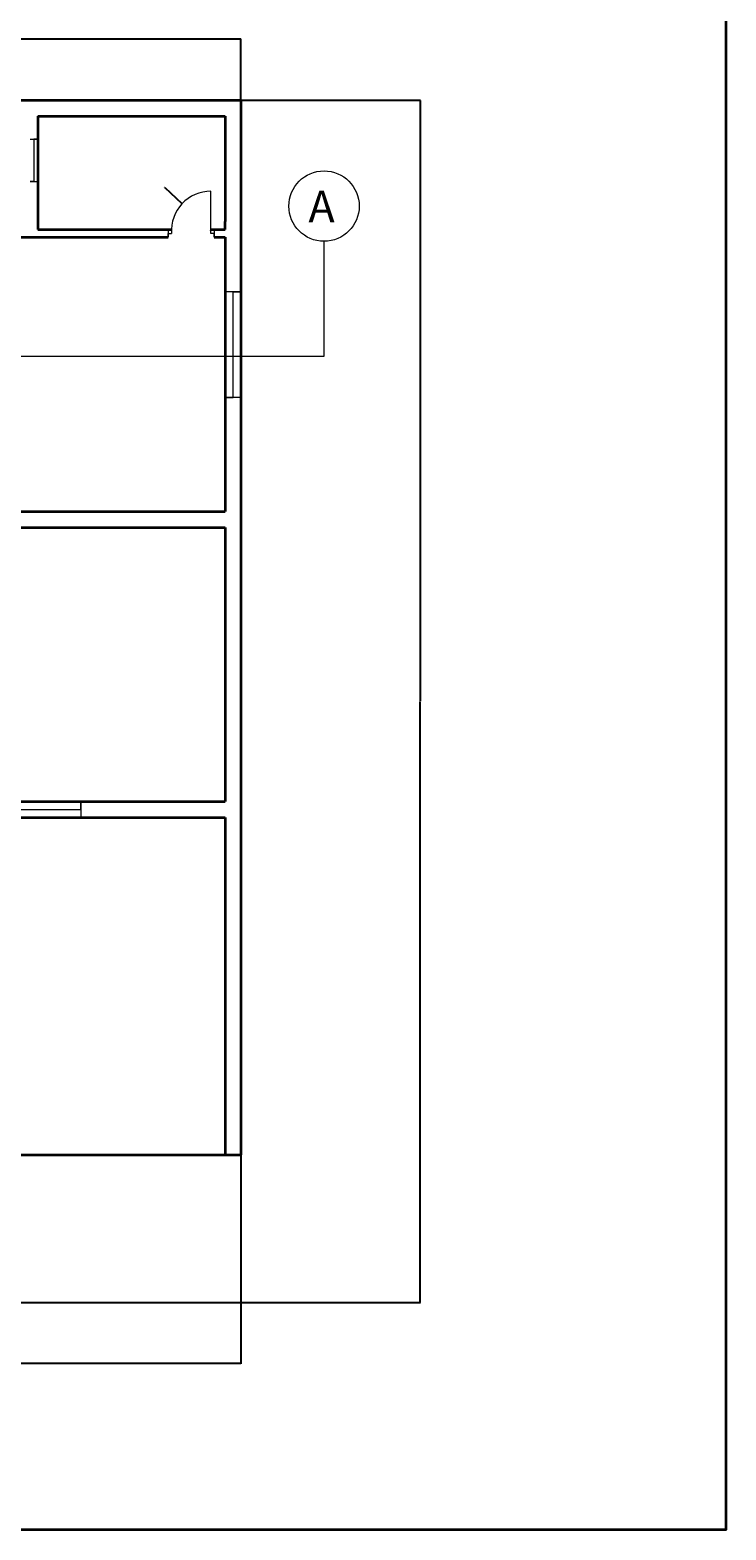
# Model space of a CAD drawing. Units: inches. Extents: x 2014 to 3678, y 870 to 2323.
# Tile 6 of 7: x 3282 to 3678, y 870 to 1723. Entities that reach past the tile are written whole.
import ezdxf

# ---------------------------------------------------------------- set-up
doc = ezdxf.new("R2010")
doc.units = ezdxf.units.IN
for name, color, linetype, lineweight in [('A-ANNO-DIMS', 2, 'Continuous', 18), ('A-ANNO-SYMB', 2, 'Continuous', 18), ('A-ANNO-TTLB', 7, 'Continuous', 35), ('A-DOOR', 3, 'Continuous', 18), ('A-GLAZ', 4, 'Continuous', 18), ('A-SITE', 8, 'Continuous', 25), ('A-WALL', 7, 'Continuous', 35)]:
    doc.layers.add(name, color=color, linetype=linetype, lineweight=lineweight)
doc.styles.get("Standard").update_dxf_attribs({"font": 'arial.ttf'})
doc.dimstyles.get("Standard").update_dxf_attribs({"dimtxt": 0.18, "dimasz": 0.18, "dimexe": 0.18, "dimexo": 0.0625, "dimgap": 0.09, "dimtad": 0, "dimtih": 1, "dimtoh": 1, "dimdec": 4, "dimzin": 0, "dimdsep": 46, "dimtxsty": 'Standard', "dimcen": 0.09, "dimadec": 0, "dimazin": 0, "dimtfac": 1, "dimtdec": 4, "dimtofl": 0, "dimtmove": 0, "dimatfit": 3, "dimfxl": 1, "dimtolj": 1, "dimtzin": 0, "dimarcsym": 0})

# ---------------------------------------------------------------- blocks, each defined once
blk = doc.blocks.new('DOOR-BATH-EAST-24')
for p, q in [((24.34, 2.25), (24.34, 26.25)), ((0, 4.5), (0, 0)), ((0, 0), (0, 2.25)), ((0, 2.25), (2, 2.25)), ((26.34, 2.25), (24.34, 2.25)), ((26.34, 4.5), (26.34, 0)), ((26.34, 0), (26.34, 2.25))]:
    blk.add_line(p, q)
blk.add_arc((24.34, 3.85), 22.4, 90, 184.10271)
blk = doc.blocks.new('WIN-60')
for p, q in [((0, 9), (0, 0)), ((60, 4.5), (60, 9)), ((60, 9), (60, 0)), ((0, 0), (0, 4.5)), ((0, 4.5), (60, 4.5))]:
    blk.add_line(p, q)
blk = doc.blocks.new('VENT-24')
for p, q in [((0, 24), (4.5, 24)), ((4.5, 24), (2.25, 24)), ((2.25, 24), (2.25, 0)), ((2.25, 0), (0, 0)), ((0, 0), (4.5, 0))]:
    blk.add_line(p, q)
blk = doc.blocks.new('*D91')
at = {"layer": 'A-ANNO-DIMS', "color": 0, "lineweight": -2, "transparency": 16777216}
for p, q in [((2848.67, 1683.23), (2848.67, 1718)), ((2848.85, 1717.82), (3125.03, 1717.82)), ((3401.99, 1717.82), (3125.82, 1717.82)), ((3402.17, 1683.23), (3402.17, 1718))]:
    blk.add_line(p, q, dxfattribs=at)
at = {"layer": 'A-ANNO-DIMS', "color": 0, "transparency": 16777216}
for points in [[(2848.85, 1717.85), (2848.85, 1717.79), (2848.67, 1717.82)], [(3401.99, 1717.85), (3401.99, 1717.79), (3402.17, 1717.82)]]:
    blk.add_solid(points, dxfattribs=at)
at = {"layer": 'Defpoints', "color": 0, "transparency": 16777216}
for p in [(3402.17, 1717.82), (2848.67, 1683.17), (3402.17, 1683.17)]:
    blk.add_point(p, dxfattribs=at)
at = {"layer": 'A-ANNO-DIMS', "color": 0, "transparency": 16777216, "insert": (3125.42, 1717.82), "char_height": 0.18, "attachment_point": 5}
blk.add_mtext('\\A1;553.5', dxfattribs=at)
blk = doc.blocks.new('*D92')
at = {"layer": 'A-ANNO-DIMS', "color": 0, "lineweight": -2, "transparency": 16777216}
for p, q in [((3402.23, 1683.17), (3504.23, 1683.17)), ((3504.05, 1682.99), (3504.05, 1341.35)), ((3504.05, 999.35), (3504.05, 1340.98)), ((3402.23, 999.17), (3504.23, 999.17))]:
    blk.add_line(p, q, dxfattribs=at)
at = {"layer": 'A-ANNO-DIMS', "color": 0, "transparency": 16777216}
for points in [[(3504.02, 1682.99), (3504.08, 1682.99), (3504.05, 1683.17)], [(3504.02, 999.35), (3504.08, 999.35), (3504.05, 999.17)]]:
    blk.add_solid(points, dxfattribs=at)
at = {"layer": 'Defpoints', "color": 0, "transparency": 16777216}
for p in [(3402.17, 1683.17), (3504.05, 1683.17), (3402.17, 999.17)]:
    blk.add_point(p, dxfattribs=at)
at = {"layer": 'A-ANNO-DIMS', "color": 0, "transparency": 16777216, "insert": (3504.05, 1341.17), "char_height": 0.18, "attachment_point": 5}
blk.add_mtext('\\A1;684', dxfattribs=at)
blk = doc.blocks.new('*D99')
at = {"layer": 'A-ANNO-DIMS', "color": 0, "lineweight": -2, "transparency": 16777216}
for p, q in [((3145.67, 999.1), (3145.67, 964.34)), ((3402.17, 999.1), (3402.17, 964.34)), ((3145.85, 964.52), (3273.53, 964.52)), ((3401.99, 964.52), (3274.32, 964.52))]:
    blk.add_line(p, q, dxfattribs=at)
at = {"layer": 'A-ANNO-DIMS', "color": 0, "transparency": 16777216}
for points in [[(3145.85, 964.55), (3145.85, 964.49), (3145.67, 964.52)], [(3401.99, 964.55), (3401.99, 964.49), (3402.17, 964.52)]]:
    blk.add_solid(points, dxfattribs=at)
at = {"layer": 'Defpoints', "color": 0, "transparency": 16777216}
for p in [(3145.67, 999.17), (3402.17, 999.17), (3402.17, 964.52)]:
    blk.add_point(p, dxfattribs=at)
at = {"layer": 'A-ANNO-DIMS', "color": 0, "transparency": 16777216, "insert": (3273.92, 964.52), "char_height": 0.18, "attachment_point": 5}
blk.add_mtext('\\A1;256.5', dxfattribs=at)
blk = doc.blocks.new('*D131')
at = {"layer": 'A-ANNO-DIMS', "color": 0, "lineweight": -2, "transparency": 16777216}
for p, q in [((3358.59, 1633.43), (3358.77, 1633.43)), ((3358.77, 1633.43), (3368.48, 1624.4)), ((3384.91, 1609.02), (3385.09, 1609.02)), ((3385, 1608.93), (3385, 1609.11))]:
    blk.add_line(p, q, dxfattribs=at)
at = {"layer": 'A-ANNO-DIMS', "color": 0, "transparency": 16777216}
blk.add_solid([(3368.5, 1624.42), (3368.46, 1624.38), (3368.61, 1624.28)], dxfattribs=at)
at = {"layer": 'Defpoints', "color": 0, "transparency": 16777216}
for p in [(3368.61, 1624.28), (3385, 1609.02)]:
    blk.add_point(p, dxfattribs=at)
at = {"layer": 'A-ANNO-DIMS', "color": 0, "transparency": 16777216, "insert": (3358.04, 1633.43), "char_height": 0.18, "attachment_point": 5}
blk.add_mtext('\\A1;R22.398', dxfattribs=at)

msp = doc.modelspace()

# ---------------------------------------------------------------- linework, layer by layer
at = {"layer": 'A-ANNO-SYMB'}
for p, q in [((3449.5026, 1537.5002), (3449.5026, 1602.9033)), ((2813.1731, 1537.5002), (3449.5026, 1537.5002))]:
    msp.add_line(p, q, dxfattribs=at)
msp.add_circle((3449.391, 1622.9101), 20.0072, dxfattribs=at)
at = {"layer": 'A-ANNO-TTLB'}
msp.add_lwpolyline([(2014.0556, 2323.3638), (3678.0069, 2323.3638), (3678.0069, 869.855), (2014.0556, 869.855)], close=True, dxfattribs=at)
at = {"layer": 'A-SITE'}
for p, q in [((3402.1718, 1083.1655), (3402.1718, 999.1655)), ((3402.1718, 999.1655), (2848.6718, 999.1655))]:
    msp.add_line(p, q, dxfattribs=at)
at = {"layer": 'A-WALL'}
for p, q in [((2848.6718, 1683.1655), (3402.1718, 1683.1655)), ((2848.6718, 1683.1655), (3402.1718, 1683.1655)), ((3402.1718, 1683.1655), (3402.1718, 1083.1655)), ((3286.6718, 1674.1655), (3393.1718, 1674.1655)), ((3286.6718, 1674.1655), (3286.6718, 1614.1655)), ((3393.1718, 1674.1655), (3393.1718, 1614.1655)), ((3286.6718, 1614.1655), (3286.6718, 1609.6655)), ((3393.1718, 1609.6655), (3393.1718, 1614.1655)), ((3216.1718, 1605.1655), (3360.6647, 1605.1655)), ((3286.6718, 1609.6655), (3362.6166, 1609.6655)), ((3385.0048, 1609.6655), (3393.1718, 1609.6655)), ((3387.0048, 1605.1655), (3393.1718, 1605.1655)), ((3393.1718, 1605.1655), (3393.1718, 1449.1655)), ((3216.1718, 1449.1655), (3393.1718, 1449.1655)), ((3216.1718, 1440.1655), (3393.1718, 1440.1655)), ((3393.1718, 1440.1655), (3393.1718, 1284.1655)), ((3216.1718, 1284.1655), (3393.1718, 1284.1655)), ((3216.1718, 1275.1655), (3393.1718, 1275.1655)), ((3393.1718, 1275.1655), (3393.1718, 1083.1655)), ((3216.1718, 1083.1655), (3402.1718, 1083.1655)), ((3393.1718, 1083.1655), (3402.1718, 1083.1655))]:
    msp.add_line(p, q, dxfattribs=at)

# ---------------------------------------------------------------- block references
at = {"layer": 'A-DOOR'}
msp.add_blockref('DOOR-BATH-EAST-24', (3360.6651, 1605.165), dxfattribs=at)
at = {"layer": 'A-GLAZ'}
for name, p in [('VENT-24', (3282.1721, 1636.939)), ('WIN-60', (3251.1162, 1275.165))]:
    msp.add_blockref(name, p, dxfattribs=at)
at = {"layer": 'A-GLAZ', "extrusion": (0, 0, -1), "zscale": -1, "rotation": 90}
msp.add_blockref('WIN-60', (-3393.1713, 1514.14), dxfattribs=at)

# ---------------------------------------------------------------- texts
at = {"layer": 'A-ANNO-SYMB', "insert": (3440.5447, 1631.6905), "char_height": 18, "attachment_point": 1}
msp.add_mtext_dynamic_manual_height_columns('A', width=78.328779, gutter_width=12.5, heights=[0], dxfattribs=at)

# ---------------------------------------------------------------- dimensions: what is measured, and where the dimension line sits
at = {"layer": 'A-ANNO-DIMS'}
for base, p1, p2, picture, middle in [((3402.1718, 1717.8155), (2848.6718, 1683.1655), (3402.1718, 1683.1655), '*D91', (3125.4218, 1717.8155)), ((3402.1718, 964.5155), (3145.6718, 999.1655), (3402.1718, 999.1655), '*D99', (3273.9218, 964.5155))]:
    dim = msp.add_linear_dim(base=base, p1=p1, p2=p2, dimstyle='Standard', override={"dimdec": 1, "dimlfac": 1, "dimrnd": 0, "dimzin": 0, "dimdsep": 46, "dimlunit": 2}, dxfattribs=at)
    dim.commit()
    dim.dimension.update_dxf_attribs({"geometry": picture, "text_midpoint": middle})
dim = msp.add_linear_dim(base=(3504.0481, 1683.1655), p1=(3402.1718, 999.1655), p2=(3402.1718, 1683.1655), angle=90, dimstyle='Standard', override={"dimdec": 0, "dimlfac": 1, "dimrnd": 0, "dimzin": 0, "dimdsep": 46, "dimlunit": 2}, dxfattribs=at)
dim.commit()
dim.dimension.update_dxf_attribs({"geometry": '*D92', "text_midpoint": (3504.0481, 1341.1655)})
dim = msp.add_radius_dim(center=(3385.0048, 1609.0179), mpoint=(3368.6106, 1624.2783), dimstyle='Standard', override={"dimdec": 3, "dimlfac": 1, "dimrnd": 0, "dimzin": 0, "dimdsep": 46, "dimlunit": 2}, dxfattribs=at)
dim.commit()
dim.dimension.update_dxf_attribs({"geometry": '*D131', "text_midpoint": (3358.0442, 1633.4346), "dimtype": 164})

doc.saveas('drawing.dxf')
